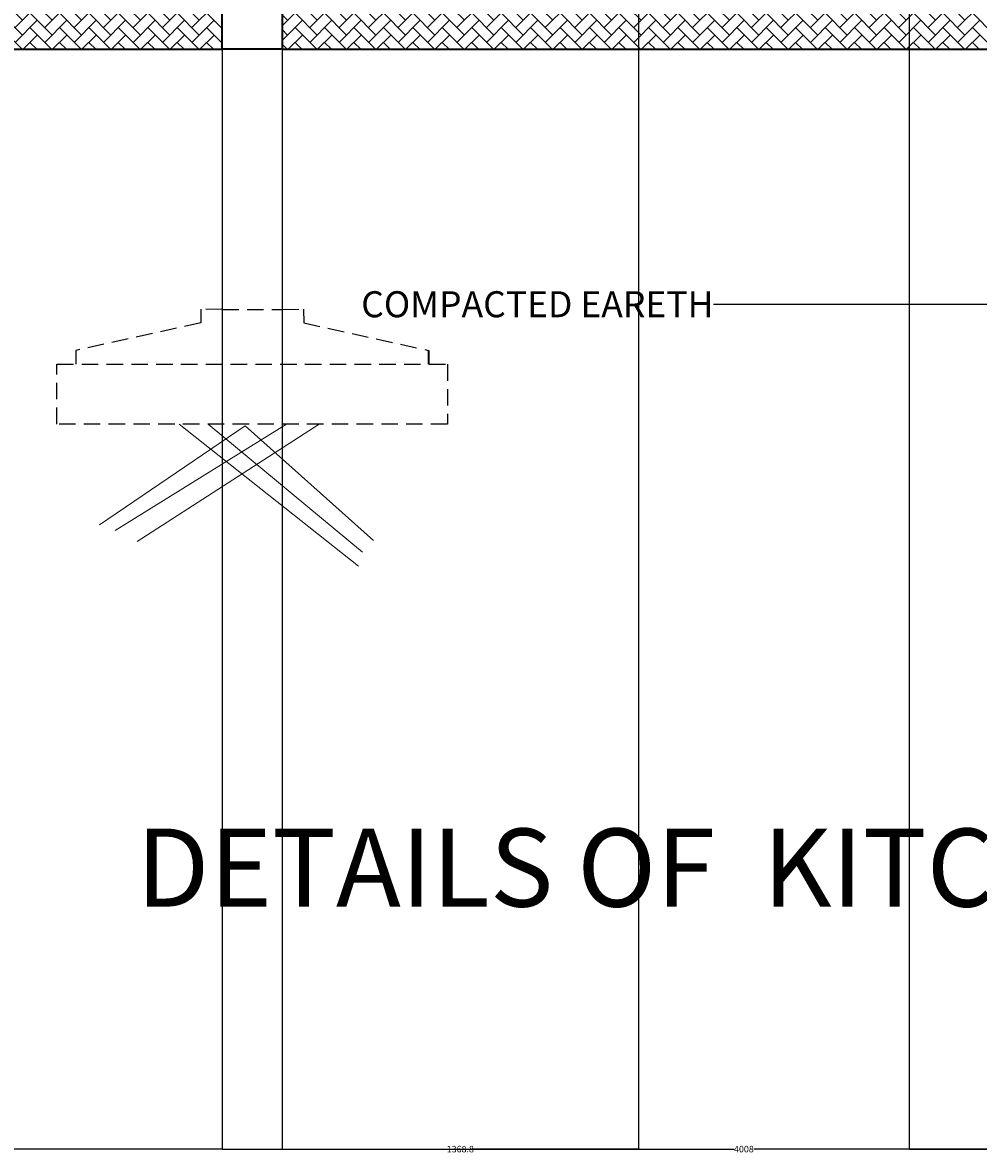
# Model space of a CAD drawing. Units: millimetres. Extents: x 1944 to 29915, y -10550 to 5909.
# Tile 11 of 24: x 15981 to 19652, y -10550 to -6203. Entities that reach past the tile are written whole.
import ezdxf
from ezdxf import colors
from ezdxf.entities.mleader import LeaderData, LeaderLine
from ezdxf.math import Vec2, Vec3

# ---------------------------------------------------------------- set-up
doc = ezdxf.new("R2010")
doc.units = ezdxf.units.MM
doc.header["$MEASUREMENT"] = 0
doc.linetypes.add('HIDDEN', pattern=[9.525, 6.35, -3.175])
for name, color, linetype, lineweight in [('A-ANNO-DIMS', 2, 'Continuous', 18), ('A-ANNO-TEXT', 7, 'Continuous', 25), ('A-FLOR-PATT', 252, 'Continuous', 13), ('A-SECT', 7, 'Continuous', 35), ('C-TOPO', 94, 'Continuous', 18), ('S-FNDN-HIDN', 1, 'HIDDEN', 25)]:
    doc.layers.add(name, color=color, linetype=linetype, lineweight=lineweight)
doc.styles.get("Standard").update_dxf_attribs({"font": 'arial.ttf'})
doc.dimstyles.get("Standard").update_dxf_attribs({"dimtxt": 25, "dimasz": 0.18, "dimexe": 0.18, "dimexo": 0.0625, "dimgap": 0.09, "dimtad": 0, "dimtih": 1, "dimtoh": 1, "dimdec": 0, "dimzin": 0, "dimdsep": 46, "dimtxsty": 'Standard', "dimcen": 0.09, "dimadec": 0, "dimazin": 0, "dimtfac": 1, "dimtdec": 0, "dimtofl": 0, "dimtmove": 0, "dimatfit": 3, "dimfxl": 1, "dimtolj": 1, "dimtzin": 0, "dimarcsym": 0})

# ---------------------------------------------------------------- blocks, each defined once
blk = doc.blocks.new('EARTH-COMPACT-SYMB')
for q in [(0, 60.9), (1053, 0)]:
    blk.add_line((559.8, 441.1), q)
blk = doc.blocks.new('*D87')
at = {"layer": 'A-ANNO-DIMS', "color": 0, "lineweight": -2, "transparency": 16777216}
for p, q in [((12344, -6305.8), (12344, -10533.3)), ((16747.8, -6305.8), (16747.8, -10533.3)), ((12344.2, -10533.1), (14508, -10533.1)), ((16747.6, -10533.1), (14583.8, -10533.1))]:
    blk.add_line(p, q, dxfattribs=at)
at = {"layer": 'A-ANNO-DIMS', "color": 0, "transparency": 16777216}
for points in [[(12344.2, -10533.1), (12344.2, -10533.1), (12344, -10533.1)], [(16747.6, -10533.1), (16747.6, -10533.1), (16747.8, -10533.1)]]:
    blk.add_solid(points, dxfattribs=at)
at = {"layer": 'Defpoints', "color": 0, "transparency": 16777216}
for p in [(12344, -6305.8), (16747.8, -6305.8), (16747.8, -10533.1)]:
    blk.add_point(p, dxfattribs=at)
at = {"layer": 'A-ANNO-DIMS', "color": 0, "transparency": 16777216, "insert": (14545.9, -10533.1), "char_height": 25, "attachment_point": 5}
blk.add_mtext('\\A1;4404', dxfattribs=at)
blk = doc.blocks.new('*D88')
at = {"layer": 'A-ANNO-DIMS', "color": 0, "lineweight": -2, "transparency": 16777216}
for p, q in [((16747.8, -6305.8), (16747.8, -10533.3)), ((20755.4, -6305.8), (20755.4, -10533.3)), ((16748, -10533.1), (18713.7, -10533.1)), ((20755.3, -10533.1), (18789.6, -10533.1))]:
    blk.add_line(p, q, dxfattribs=at)
at = {"layer": 'A-ANNO-DIMS', "color": 0, "transparency": 16777216}
for points in [[(16748, -10533.1), (16748, -10533.1), (16747.8, -10533.1)], [(20755.3, -10533.1), (20755.3, -10533.1), (20755.4, -10533.1)]]:
    blk.add_solid(points, dxfattribs=at)
at = {"layer": 'Defpoints', "color": 0, "transparency": 16777216}
for p in [(16747.8, -6305.8), (20755.4, -6305.8), (20755.4, -10533.1)]:
    blk.add_point(p, dxfattribs=at)
at = {"layer": 'A-ANNO-DIMS', "color": 0, "transparency": 16777216, "insert": (18751.6, -10533.1), "char_height": 25, "attachment_point": 5}
blk.add_mtext('\\A1;4008', dxfattribs=at)
blk = doc.blocks.new('*D97')
at = {"layer": 'A-ANNO-DIMS', "color": 0, "lineweight": -2, "transparency": 16777216}
for p, q in [((16977.8, -5945.8), (16977.8, -10533.3)), ((18346.6, -5945.8), (18346.6, -10533.3)), ((16978, -10533.1), (17611.4, -10533.1)), ((18346.5, -10533.1), (17713.1, -10533.1))]:
    blk.add_line(p, q, dxfattribs=at)
at = {"layer": 'A-ANNO-DIMS', "color": 0, "transparency": 16777216}
for points in [[(16978, -10533.1), (16978, -10533.1), (16977.8, -10533.1)], [(18346.5, -10533.1), (18346.5, -10533.1), (18346.6, -10533.1)]]:
    blk.add_solid(points, dxfattribs=at)
at = {"layer": 'Defpoints', "color": 0, "transparency": 16777216}
for p in [(16977.8, -5945.8), (18346.6, -5945.8), (18346.6, -10533.1)]:
    blk.add_point(p, dxfattribs=at)
at = {"layer": 'A-ANNO-DIMS', "color": 0, "transparency": 16777216, "insert": (17662.2, -10533.1), "char_height": 25, "attachment_point": 5}
blk.add_mtext('\\A1;1368.8', dxfattribs=at)
blk = doc.blocks.new('*D98')
at = {"layer": 'A-ANNO-DIMS', "color": 0, "lineweight": -2, "transparency": 16777216}
for p, q in [((19386.6, -5945.8), (19386.6, -10533.3)), ((20755.4, -5945.8), (20755.4, -10533.3)), ((19386.8, -10533.1), (20020.2, -10533.1)), ((20755.3, -10533.1), (20121.9, -10533.1))]:
    blk.add_line(p, q, dxfattribs=at)
at = {"layer": 'A-ANNO-DIMS', "color": 0, "transparency": 16777216}
for points in [[(19386.8, -10533.1), (19386.8, -10533.1), (19386.6, -10533.1)], [(20755.3, -10533.1), (20755.3, -10533.1), (20755.4, -10533.1)]]:
    blk.add_solid(points, dxfattribs=at)
at = {"layer": 'Defpoints', "color": 0, "transparency": 16777216}
for p in [(19386.6, -5945.8), (20755.4, -5945.8), (20755.4, -10533.1)]:
    blk.add_point(p, dxfattribs=at)
at = {"layer": 'A-ANNO-DIMS', "color": 0, "transparency": 16777216, "insert": (20071, -10533.1), "char_height": 25, "attachment_point": 5}
blk.add_mtext('\\A1;1368.8', dxfattribs=at)

msp = doc.modelspace()

# ---------------------------------------------------------------- hatches: boundary and pattern name
at = {"layer": 'A-FLOR-PATT'}
h = msp.add_hatch(dxfattribs=at)
h.set_pattern_fill('AR-HBONE', color=256, scale=10)
h.paths.add_polyline_path([(12573.981, -6073.852), (12573.981, -6305.752), (16747.828, -6305.752), (16747.828, -6073.852)])
h = msp.add_hatch(dxfattribs=at)
h.set_pattern_fill('AR-HBONE', color=256, scale=10)
h.paths.add_polyline_path([(20755.45, -6073.852), (16977.828, -6073.852), (16977.828, -6305.752), (20755.45, -6305.752)])

# ---------------------------------------------------------------- linework, layer by layer
at = {"layer": 'A-SECT'}
for p, q in [((12573.981, -6305.752), (16747.828, -6305.752)), ((16977.828, -6305.752), (20755.45, -6305.752)), ((17540.452, -7463.338), (17540.452, -7516.218))]:
    msp.add_line(p, q, dxfattribs=at)
msp.add_lwpolyline([(16747.828, -5945.752), (16977.828, -5945.752), (16977.828, -6305.752), (16747.828, -6305.752)], close=True, dxfattribs=at)
at = {"layer": 'C-TOPO'}
for p, q in [((16994.892, -7746.218), (16336.593, -8155.847)), ((17119.846, -7746.218), (16420.405, -8196.963)), ((16581.931, -7746.218), (17270.706, -8292.9)), ((16693.172, -7746.218), (17285.945, -8238.079))]:
    msp.add_line(p, q, dxfattribs=at)
at = {"layer": 'S-FNDN-HIDN', "ltscale": 10}
for p, q in [((16747.828, -6305.752), (16747.828, -7305.752)), ((16977.828, -6305.752), (16977.828, -7305.752)), ((16665.799, -7304.748), (16665.157, -7357.264)), ((16747.828, -7305.752), (16665.799, -7304.748)), ((16747.828, -7305.752), (16977.828, -7305.752)), ((16977.828, -7305.752), (17059.857, -7304.748)), ((17059.857, -7304.748), (17060.5, -7357.264)), ((16665.157, -7357.264), (16185.204, -7463.338)), ((17060.5, -7357.264), (17540.452, -7463.338)), ((16185.204, -7463.338), (16185.204, -7516.218))]:
    msp.add_line(p, q, dxfattribs=at)
msp.add_lwpolyline([(16112.828, -7516.218), (17612.828, -7516.218), (17612.828, -7746.218), (16112.828, -7746.218)], close=True, dxfattribs=at)

# ---------------------------------------------------------------- block references
at = {"layer": 'C-TOPO'}
msp.add_blockref('EARTH-COMPACT-SYMB', (16275.64, -8193.917), dxfattribs=at)

# ---------------------------------------------------------------- texts
at = {"layer": 'A-ANNO-TEXT'}
msp.add_text('DETAILS OF  KITCHEN', height=300, dxfattribs=at).set_placement((16416.91, -9601.103))

# ---------------------------------------------------------------- dimensions: what is measured, and where the dimension line sits
at = {"layer": 'A-ANNO-DIMS'}
for base, p1, p2, override, picture, middle in [((18346.639, -10533.115), (16977.828, -5945.752), (18346.639, -5945.752), {"dimdec": 1, "dimlfac": 1, "dimrnd": 0, "dimzin": 0, "dimdsep": 46, "dimlunit": 2}, '*D97', (17662.234, -10533.115)), ((20755.45, -10533.115), (19386.639, -5945.752), (20755.45, -5945.752), {"dimdec": 1, "dimlfac": 1, "dimrnd": 0, "dimzin": 0, "dimdsep": 46, "dimlunit": 2}, '*D98', (20071.044, -10533.115)), ((16747.828, -10533.115), (12343.981, -6305.752), (16747.828, -6305.752), {"dimdec": 0, "dimlfac": 1, "dimrnd": 0, "dimzin": 0, "dimdsep": 46, "dimlunit": 2}, '*D87', (14545.905, -10533.115)), ((20755.45, -10533.115), (16747.828, -6305.752), (20755.45, -6305.752), {"dimdec": 0, "dimlfac": 1, "dimrnd": 0, "dimzin": 0, "dimdsep": 46, "dimlunit": 2}, '*D88', (18751.639, -10533.115))]:
    dim = msp.add_linear_dim(base=base, p1=p1, p2=p2, dimstyle='Standard', override=override, dxfattribs=at)
    dim.commit()
    dim.dimension.update_dxf_attribs({"geometry": picture, "text_midpoint": middle})

# ---------------------------------------------------------------- leaders
at = {"layer": 'A-ANNO-TEXT'}
ml = msp.add_multileader_mtext('Standard', dxfattribs=at)
ml.set_content('COMPACTED EARETH ', color=256)
ml.set_leader_properties()
ml.build(insert=Vec2(0, 0))
ml.multileader.update_dxf_attribs({"dogleg_length": 568.936, "arrow_head_size": 100})
ctx = ml.context
ctx.base_point, ctx.char_height, ctx.arrow_head_size, ctx.landing_gap_size, ctx.plane_origin = Vec3(17154.841, -7286.495), 100, 100, 0.09, Vec3(19203.765, -7286.495)
ctx.text_align_type = 2
notes = []
notes.append((ctx, [(0, (1, 1, 0), (19203.765, -7286.495), (-1, 0), 568.936, [(0, [(20352.82, -6305.752), (20352.82, -7286.495)], 0, [])])]))
ctx.mtext.insert, ctx.mtext.alignment, ctx.mtext.flow_direction = Vec3(18634.74, -7235.642), 3, 5
for ctx, leaders in notes:
    for number, flags, end, landing, length, lines in leaders:
        leader = LeaderData()
        leader.index, (leader.has_last_leader_line, leader.has_dogleg_vector, leader.attachment_direction) = number, flags
        leader.last_leader_point, leader.dogleg_vector, leader.dogleg_length = Vec3(end), Vec3(landing), length
        for number, points, colour, breaks in lines:
            line = LeaderLine()
            line.index, line.vertices, line.color, line.breaks = number, Vec3.list(points), colors.encode_raw_color(colour), breaks
            leader.lines.append(line)
        ctx.leaders.append(leader)

doc.saveas('drawing.dxf')
